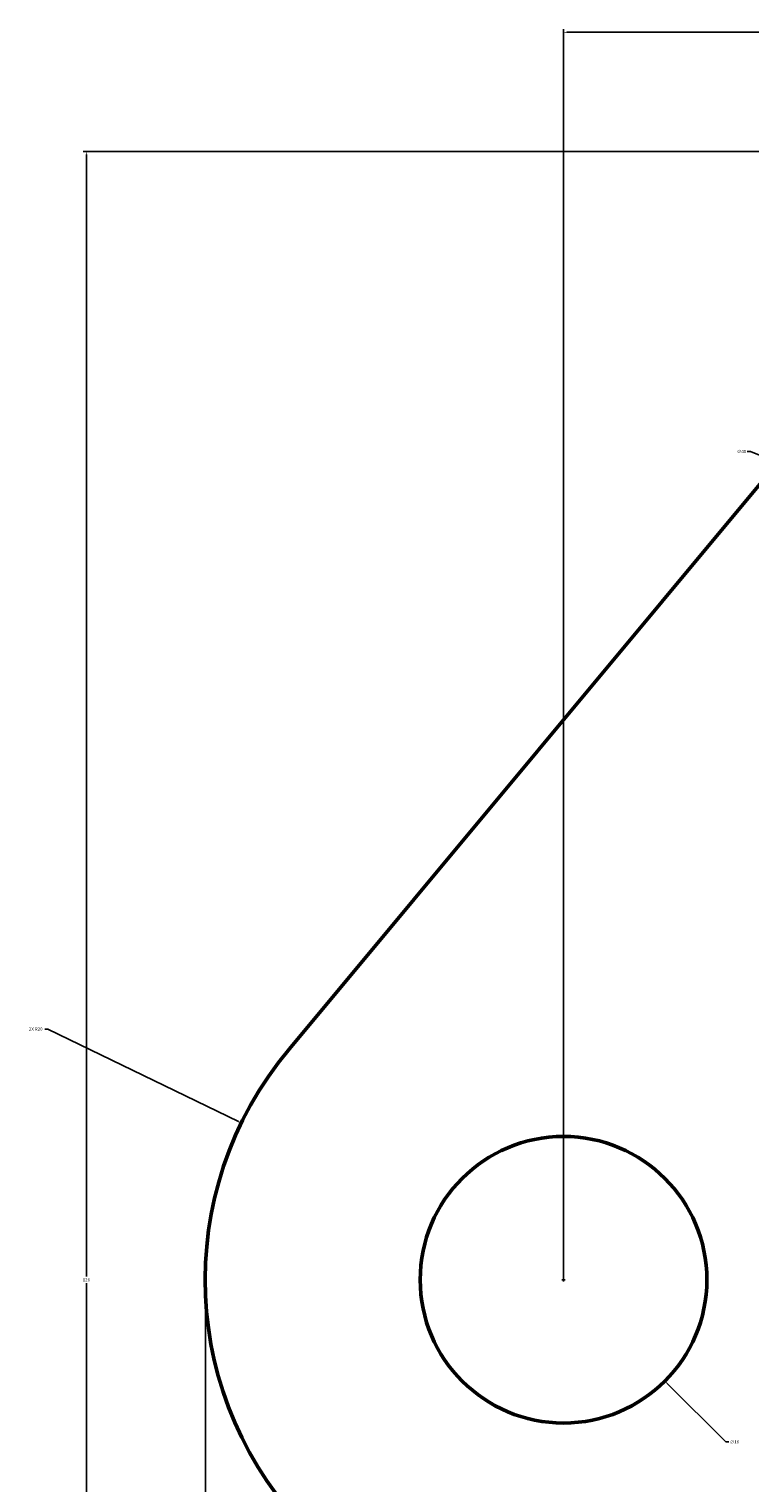
# Model space of a CAD drawing. Units: inches. Extents: x -11 to 126, y -62 to 82.
# Tile 6 of 10: x -11 to 30, y 1 to 82. Entities that reach past the tile are written whole.
import ezdxf

# ---------------------------------------------------------------- set-up
doc = ezdxf.new("R2010")
doc.units = ezdxf.units.IN
doc.header["$MEASUREMENT"] = 0
doc.layers.add('M-DIMS', color=2, linetype='Continuous', lineweight=18)
doc.layers.add('M-OUTL', color=7, linetype='Continuous', lineweight=50)
doc.styles.get("Standard").update_dxf_attribs({"font": 'arial.ttf'})
doc.dimstyles.get("Standard").update_dxf_attribs({"dimtxt": 0.18, "dimasz": 0.18, "dimexe": 0.18, "dimexo": 0.0625, "dimgap": 0.09, "dimtad": 0, "dimtih": 1, "dimtoh": 1, "dimdec": 4, "dimzin": 0, "dimdsep": 46, "dimtxsty": 'Standard', "dimcen": 0.09, "dimadec": 0, "dimazin": 0, "dimtfac": 1, "dimtdec": 4, "dimtofl": 0, "dimtmove": 0, "dimatfit": 3, "dimfxl": 1, "dimtolj": 1, "dimtzin": 0, "dimarcsym": 0})

# ---------------------------------------------------------------- blocks, each defined once
blk = doc.blocks.new('*D5')
at = {"layer": 'Defpoints', "color": 0, "transparency": 16777216}
for p in [(119.232, 12.354), (-0.749, 11.479), (119.232, -57.296)]:
    blk.add_point(p, dxfattribs=at)
at = {"layer": 'M-DIMS', "color": 0, "lineweight": -2, "transparency": 16777216}
for p, q in [((119.232, 12.292), (119.232, -57.476)), ((-0.749, 11.416), (-0.749, -57.476)), ((-0.569, -57.296), (58.786, -57.296)), ((119.052, -57.296), (59.696, -57.296))]:
    blk.add_line(p, q, dxfattribs=at)
at = {"layer": 'M-DIMS', "color": 0, "transparency": 16777216}
for points in [[(-0.569, -57.266), (-0.569, -57.326), (-0.749, -57.296)], [(119.052, -57.266), (119.052, -57.326), (119.232, -57.296)]]:
    blk.add_solid(points, dxfattribs=at)
at = {"layer": 'M-DIMS', "color": 0, "transparency": 16777216, "insert": (59.241, -57.296), "char_height": 0.18, "attachment_point": 5}
blk.add_mtext('\\A1;119.98', dxfattribs=at)
blk = doc.blocks.new('*D6')
at = {"layer": 'Defpoints', "color": 0, "transparency": 16777216}
for p in [(-7.399, 75.354), (59.232, 75.354), (59.232, -50.646)]:
    blk.add_point(p, dxfattribs=at)
at = {"layer": 'M-DIMS', "color": 0, "lineweight": -2, "transparency": 16777216}
for p, q in [((59.169, 75.354), (-7.579, 75.354)), ((-7.399, 75.174), (-7.399, 12.536)), ((-7.399, -50.466), (-7.399, 12.172)), ((59.169, -50.646), (-7.579, -50.646))]:
    blk.add_line(p, q, dxfattribs=at)
at = {"layer": 'M-DIMS', "color": 0, "transparency": 16777216}
for points in [[(-7.429, 75.174), (-7.369, 75.174), (-7.399, 75.354)], [(-7.429, -50.466), (-7.369, -50.466), (-7.399, -50.646)]]:
    blk.add_solid(points, dxfattribs=at)
at = {"layer": 'M-DIMS', "color": 0, "transparency": 16777216, "insert": (-7.399, 12.354), "char_height": 0.18, "attachment_point": 5}
blk.add_mtext('\\A1;126', dxfattribs=at)
blk = doc.blocks.new('*D7')
at = {"layer": 'Defpoints', "color": 0, "transparency": 16777216}
for p in [(59.232, 82.004), (59.232, 46.354), (19.232, 12.354)]:
    blk.add_point(p, dxfattribs=at)
at = {"layer": 'M-DIMS', "color": 0, "lineweight": -2, "transparency": 16777216}
for p, q in [((19.232, 12.417), (19.232, 82.184)), ((19.412, 82.004), (39.009, 82.004)), ((59.052, 82.004), (39.454, 82.004)), ((59.232, 46.417), (59.232, 82.184))]:
    blk.add_line(p, q, dxfattribs=at)
at = {"layer": 'M-DIMS', "color": 0, "transparency": 16777216}
for points in [[(19.412, 82.034), (19.412, 81.974), (19.232, 82.004)], [(59.052, 82.034), (59.052, 81.974), (59.232, 82.004)]]:
    blk.add_solid(points, dxfattribs=at)
at = {"layer": 'M-DIMS', "color": 0, "transparency": 16777216, "insert": (39.232, 82.004), "char_height": 0.18, "attachment_point": 5}
blk.add_mtext('\\A1;40', dxfattribs=at)
blk = doc.blocks.new('*D14')
at = {"layer": 'Defpoints', "color": 0, "transparency": 16777216}
for p in [(40.754, 54.008), (77.709, 38.701)]:
    blk.add_point(p, dxfattribs=at)
at = {"layer": 'M-DIMS', "color": 0, "lineweight": -2, "transparency": 16777216}
for p, q in [((29.487, 58.6), (29.667, 58.6)), ((29.667, 58.6), (40.588, 54.077)), ((59.142, 46.354), (59.322, 46.354)), ((59.232, 46.264), (59.232, 46.444))]:
    blk.add_line(p, q, dxfattribs=at)
at = {"layer": 'M-DIMS', "color": 0, "transparency": 16777216}
blk.add_solid([(40.599, 54.105), (40.576, 54.049), (40.754, 54.008)], dxfattribs=at)
at = {"layer": 'M-DIMS', "color": 0, "transparency": 16777216, "insert": (29.171, 58.6), "char_height": 0.18, "attachment_point": 5}
blk.add_mtext('\\A1;∅40', dxfattribs=at)
blk = doc.blocks.new('*D16')
at = {"layer": 'Defpoints', "color": 0, "transparency": 16777216}
for p in [(1.246, 21.102), (19.232, 12.354)]:
    blk.add_point(p, dxfattribs=at)
at = {"layer": 'M-DIMS', "color": 0, "lineweight": -2, "transparency": 16777216}
for p, q in [((-9.725, 26.351), (-9.545, 26.351)), ((-9.545, 26.351), (1.084, 21.181)), ((19.142, 12.354), (19.322, 12.354)), ((19.232, 12.264), (19.232, 12.444))]:
    blk.add_line(p, q, dxfattribs=at)
at = {"layer": 'M-DIMS', "color": 0, "transparency": 16777216}
blk.add_solid([(1.097, 21.208), (1.071, 21.154), (1.246, 21.102)], dxfattribs=at)
at = {"layer": 'M-DIMS', "color": 0, "transparency": 16777216, "insert": (-10.225, 26.351), "char_height": 0.18, "attachment_point": 5}
blk.add_mtext('\\A1;2X R20', dxfattribs=at)
blk = doc.blocks.new('*D18')
at = {"layer": 'Defpoints', "color": 0, "transparency": 16777216}
for p in [(13.575, 18.011), (24.888, 6.698)]:
    blk.add_point(p, dxfattribs=at)
at = {"layer": 'M-DIMS', "color": 0, "lineweight": -2, "transparency": 16777216}
for p, q in [((19.142, 12.354), (19.322, 12.354)), ((19.232, 12.264), (19.232, 12.444)), ((28.283, 3.303), (25.016, 6.57)), ((28.463, 3.303), (28.283, 3.303))]:
    blk.add_line(p, q, dxfattribs=at)
at = {"layer": 'M-DIMS', "color": 0, "transparency": 16777216}
blk.add_solid([(25.037, 6.591), (24.995, 6.549), (24.888, 6.698)], dxfattribs=at)
at = {"layer": 'M-DIMS', "color": 0, "transparency": 16777216, "insert": (28.779, 3.303), "char_height": 0.18, "attachment_point": 5}
blk.add_mtext('\\A1;∅16', dxfattribs=at)

msp = doc.modelspace()

# ---------------------------------------------------------------- linework, layer by layer
at = {"layer": 'M-OUTL'}
msp.add_line((3.94, 25.244), (36.676, 64.582), dxfattribs=at)
msp.add_circle((19.232, 12.354), 8, dxfattribs=at)
msp.add_arc((19.232, 12.354), 20, 139.87157, 225.14721, dxfattribs=at)

# ---------------------------------------------------------------- dimensions: what is measured, and where the dimension line sits
at = {"layer": 'M-DIMS'}
for base, p1, p2, override, picture, middle in [((59.232, 82.004), (19.232, 12.354), (59.232, 46.354), {"dimdec": 0, "dimlfac": 1, "dimrnd": 0, "dimzin": 0, "dimdsep": 46, "dimlunit": 2}, '*D7', (39.232, 82.004)), ((119.232, -57.296), (-0.749, 11.479), (119.232, 12.354), {"dimdec": 2, "dimlfac": 1, "dimrnd": 0, "dimzin": 0, "dimdsep": 46, "dimlunit": 2}, '*D5', (59.241, -57.296))]:
    dim = msp.add_linear_dim(base=base, p1=p1, p2=p2, dimstyle='Standard', override=override, dxfattribs=at)
    dim.commit()
    dim.dimension.update_dxf_attribs({"geometry": picture, "text_midpoint": middle})
dim = msp.add_linear_dim(base=(-7.399, 75.354), p1=(59.232, -50.646), p2=(59.232, 75.354), angle=90, dimstyle='Standard', override={"dimdec": 0, "dimlfac": 1, "dimrnd": 0, "dimzin": 0, "dimdsep": 46, "dimlunit": 2}, dxfattribs=at)
dim.commit()
dim.dimension.update_dxf_attribs({"geometry": '*D6', "text_midpoint": (-7.399, 12.354)})
for p1, p2, picture, middle in [((77.709, 38.701), (40.754, 54.008), '*D14', (29.171, 58.6)), ((13.575, 18.011), (24.888, 6.698), '*D18', (28.779, 3.303))]:
    dim = msp.add_diameter_dim_2p(p1=p1, p2=p2, dimstyle='Standard', override={"dimdec": 0, "dimlfac": 1, "dimrnd": 0, "dimzin": 0, "dimdsep": 46, "dimlunit": 2}, dxfattribs=at)
    dim.commit()
    dim.dimension.update_dxf_attribs({"geometry": picture, "text_midpoint": middle, "dimtype": 163})
dim = msp.add_radius_dim(center=(19.232, 12.354), mpoint=(1.246, 21.102), text='2X <>', dimstyle='Standard', override={"dimdec": 0, "dimlfac": 1, "dimrnd": 0, "dimzin": 0, "dimdsep": 46, "dimlunit": 2}, dxfattribs=at)
dim.commit()
dim.dimension.update_dxf_attribs({"geometry": '*D16', "text_midpoint": (-10.225, 26.351), "dimtype": 164})

doc.saveas('drawing.dxf')
